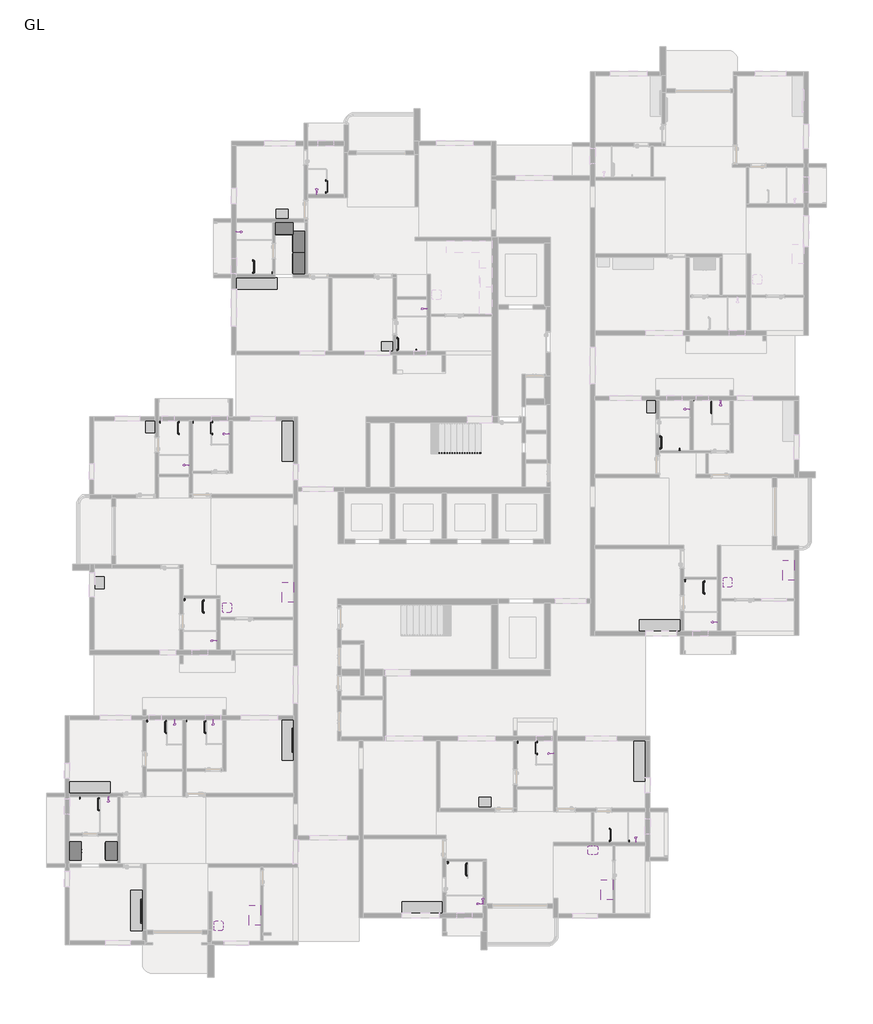
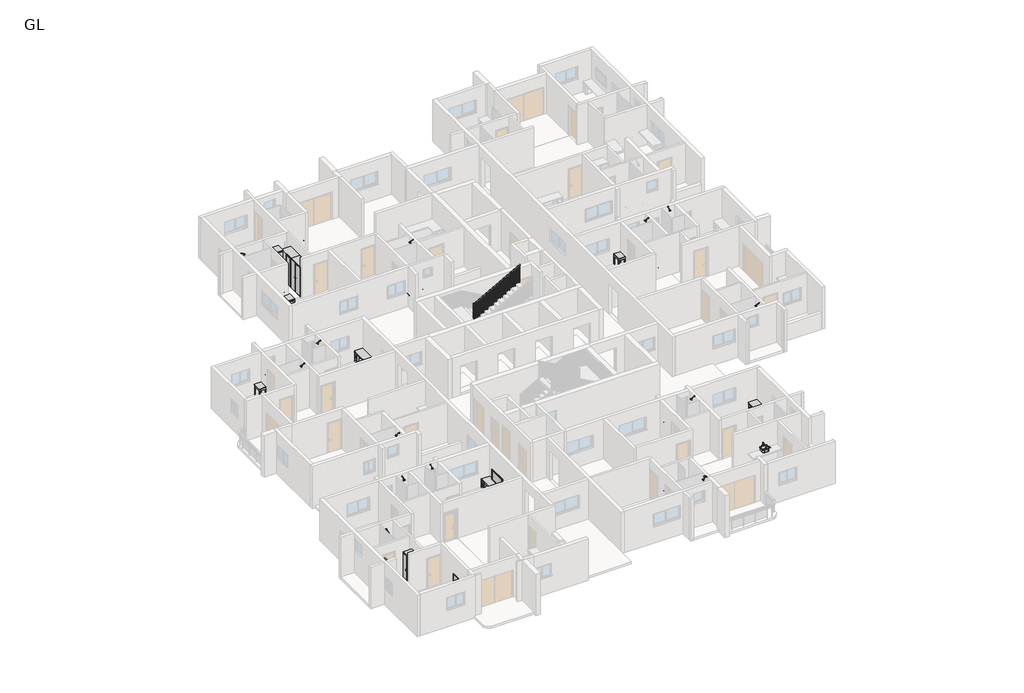
# One storey, part 13 of 14: 50 flow terminals, 23 furniture elements, 4 proxies, 1 railing.
"""IFC4 building model written with IfcOpenShell, lengths in millimetres."""

from ifc_helpers import new_model, si_unit, frame, origin, place, context, project, spatial, polyline, outline, extrude, faceted_brep, transform, mapped, element, save
from components import cook_top_2_0915_x_500mm_892363c5, flow_terminal_f629513f, grab_rail_horizontal_grab_bar_horizontal_f73a8c0c, grab_rail_vertical_grab_rail_vertical_969059c8, plumbing_fixtures_shower_head_metal_shower_head_9404fff0, furniture_8acf2248, escritorio_de_estudiante_de_600x740mm_600_x_460_x_740mm_3f482482, furniture_0b97a49d, furniture_eb486d47, wardrobe_family_wardrobe_large_408d0eaf, wardrobe_family_wardrobe_small_46214fc7

model = new_model("IFC4")

# Units and contexts
model_context = context("Model", 3, world=origin())
ifc_project = project(units=[si_unit("LENGTHUNIT", "METRE", prefix="MILLI")], contexts=[model_context])

# Site, building, storey
site = spatial("IfcSite", under=ifc_project)
building = spatial("IfcBuilding", under=site)
storey = spatial("IfcBuildingStorey", under=building, Name="GL", Elevation=0.0)

# Proxies
placement = place(None, origin())
cook_top_2_0915_x_500mm_shape = cook_top_2_0915_x_500mm_892363c5(model_context)
element("IfcBuildingElementProxy", 1, Name="Cook_Top_(2) : 0915 x 500mm", ObjectType="Cook_Top_(2) : 0915 x 500mm", at=placement, inside=storey, context=model_context, shape_type="MappedRepresentation", body=[
    mapped(cook_top_2_0915_x_500mm_shape, transform((-7432.3172689, 57616.4127724, 457.2), x_axis=(0.0, 1.0, 0.0), y_axis=(-1.0, 0.0, 0.0), z_axis=(0.0, 0.0, 1.0))),
])
element("IfcBuildingElementProxy", 2, Name="Cook_Top_(2) : 0915 x 500mm", ObjectType="Cook_Top_(2) : 0915 x 500mm", at=placement, inside=storey, context=model_context, shape_type="MappedRepresentation", body=[
    mapped(cook_top_2_0915_x_500mm_shape, transform((10113.003694, 58890.1105424, 457.2), x_axis=(0.0, 1.0, 0.0), y_axis=(-1.0, 0.0, 0.0), z_axis=(0.0, 0.0, 1.0))),
])
element("IfcBuildingElementProxy", 3, Name="Cook_Top_(2) : 0915 x 500mm", ObjectType="Cook_Top_(2) : 0915 x 500mm", at=placement, inside=storey, context=model_context, shape_type="MappedRepresentation", body=[
    mapped(cook_top_2_0915_x_500mm_shape, transform((19166.6969726, 74807.6047412, 457.2), x_axis=(0.0, 1.0, 0.0), y_axis=(-1.0, 0.0, 0.0), z_axis=(0.0, 0.0, 1.0))),
])
element("IfcBuildingElementProxy", 4, Name="Cook_Top_(2) : 0915 x 500mm", ObjectType="Cook_Top_(2) : 0915 x 500mm", at=placement, inside=storey, context=model_context, shape_type="MappedRepresentation", body=[
    mapped(cook_top_2_0915_x_500mm_shape, transform((-5780.9131346, 73713.6131717, 457.2), x_axis=(0.0, 1.0, 0.0), y_axis=(-1.0, 0.0, 0.0), z_axis=(0.0, 0.0, 1.0))),
])

# Flow terminals
flow_terminal_shape = flow_terminal_f629513f(model_context)
element("IfcFlowTerminal", 5, at=placement, inside=storey, context=model_context, shape_type="MappedRepresentation", body=[
    mapped(flow_terminal_shape, transform((-9284.2164285, 57077.0304817, 762.0), x_axis=(0.0, 1.0, 0.0), y_axis=(-1.0, 0.0, 0.0), z_axis=(0.0, 0.0, 1.0))),
])
element("IfcFlowTerminal", 6, at=placement, inside=storey, context=model_context, shape_type="MappedRepresentation", body=[
    mapped(flow_terminal_shape, transform((16090.1365547, 74192.2476782, 762.0), x_axis=(0.0, 1.0, 0.0), y_axis=(-1.0, 0.0, 0.0), z_axis=(0.0, 0.0, 1.0))),
])
element("IfcFlowTerminal", 7, at=placement, inside=storey, context=model_context, shape_type="MappedRepresentation", body=[
    mapped(flow_terminal_shape, transform((-8863.3729222, 72934.9514566, 762.0), x_axis=(0.0, 1.0, 0.0), y_axis=(-1.0, 0.0, 0.0), z_axis=(0.0, 0.0, 1.0))),
])
element("IfcFlowTerminal", 8, at=placement, inside=storey, context=model_context, shape_type="MappedRepresentation", body=[
    mapped(flow_terminal_shape, transform((9390.7046133, 60899.7565929, 762.0), x_axis=(1.0, 0.0, 0.0), y_axis=(0.0, 1.0, 0.0), z_axis=(0.0, 0.0, 1.0))),
])
grab_rail_horizontal_grab_bar_horizontal_shape = grab_rail_horizontal_grab_bar_horizontal_f73a8c0c(model_context)
element("IfcFlowTerminal", 9, ObjectType="Grab Rail - Horizontal : Grab Bar Horizontal", at=placement, inside=storey, context=model_context, shape_type="MappedRepresentation", body=[
    mapped(grab_rail_horizontal_grab_bar_horizontal_shape, transform((-15187.4698866, 64009.4643641, 0.0), x_axis=(0.0, 1.0, 0.0), y_axis=(-1.0, 0.0, 0.0), z_axis=(0.0, 0.0, 1.0))),
])
element("IfcFlowTerminal", 10, ObjectType="Grab Rail - Horizontal : Grab Bar Horizontal", at=placement, inside=storey, context=model_context, shape_type="MappedRepresentation", body=[
    mapped(grab_rail_horizontal_grab_bar_horizontal_shape, transform((-11834.397169, 67857.3290817, 0.0), x_axis=(0.0, 1.0, 0.0), y_axis=(-1.0, 0.0, 0.0), z_axis=(0.0, 0.0, 1.0))),
])
element("IfcFlowTerminal", 11, ObjectType="Grab Rail - Horizontal : Grab Bar Horizontal", at=placement, inside=storey, context=model_context, shape_type="MappedRepresentation", body=[
    mapped(grab_rail_horizontal_grab_bar_horizontal_shape, transform((-9878.597169, 67857.3290817, 0.0), x_axis=(0.0, 1.0, 0.0), y_axis=(-1.0, 0.0, 0.0), z_axis=(0.0, 0.0, 1.0))),
])
element("IfcFlowTerminal", 12, ObjectType="Grab Rail - Horizontal : Grab Bar Horizontal", at=placement, inside=storey, context=model_context, shape_type="MappedRepresentation", body=[
    mapped(grab_rail_horizontal_grab_bar_horizontal_shape, transform((6641.3567087, 66815.1785086, 0.0), x_axis=(0.0, 1.0, 0.0), y_axis=(-1.0, 0.0, 0.0), z_axis=(0.0, 0.0, 1.0))),
])
element("IfcFlowTerminal", 13, ObjectType="Grab Rail - Horizontal : Grab Bar Horizontal", at=placement, inside=storey, context=model_context, shape_type="MappedRepresentation", body=[
    mapped(grab_rail_horizontal_grab_bar_horizontal_shape, transform((10234.603694, 60775.9743275, 0.0), x_axis=(0.0, -1.0, 0.0), y_axis=(1.0, 0.0, 0.0), z_axis=(0.0, 0.0, 1.0))),
])
element("IfcFlowTerminal", 14, ObjectType="Grab Rail - Horizontal : Grab Bar Horizontal", at=placement, inside=storey, context=model_context, shape_type="MappedRepresentation", body=[
    mapped(grab_rail_horizontal_grab_bar_horizontal_shape, transform((3159.1144026, 60758.453971, 0.0), x_axis=(0.0, 1.0, 0.0), y_axis=(-1.0, 0.0, 0.0), z_axis=(0.0, 0.0, 1.0))),
])
element("IfcFlowTerminal", 15, ObjectType="Grab Rail - Horizontal : Grab Bar Horizontal", at=placement, inside=storey, context=model_context, shape_type="MappedRepresentation", body=[
    mapped(grab_rail_horizontal_grab_bar_horizontal_shape, transform((14986.6163556, 74808.9935622, 0.0), x_axis=(0.0, 1.0, 0.0), y_axis=(-1.0, 0.0, 0.0), z_axis=(0.0, 0.0, 1.0))),
])
element("IfcFlowTerminal", 16, ObjectType="Grab Rail - Horizontal : Grab Bar Horizontal", at=placement, inside=storey, context=model_context, shape_type="MappedRepresentation", body=[
    mapped(grab_rail_horizontal_grab_bar_horizontal_shape, transform((12762.5764579, 80324.0622292, 0.0), x_axis=(0.0, -1.0, 0.0), y_axis=(1.0, 0.0, 0.0), z_axis=(0.0, 0.0, 1.0))),
])
element("IfcFlowTerminal", 17, ObjectType="Grab Rail - Horizontal : Grab Bar Horizontal", at=placement, inside=storey, context=model_context, shape_type="MappedRepresentation", body=[
    mapped(grab_rail_horizontal_grab_bar_horizontal_shape, transform((15380.1764579, 83771.3835622, 0.0), x_axis=(0.0, 1.0, 0.0), y_axis=(-1.0, 0.0, 0.0), z_axis=(0.0, 0.0, 1.0))),
])
element("IfcFlowTerminal", 18, ObjectType="Grab Rail - Horizontal : Grab Bar Horizontal", at=placement, inside=storey, context=model_context, shape_type="MappedRepresentation", body=[
    mapped(grab_rail_horizontal_grab_bar_horizontal_shape, transform((-7539.4662192, 89078.9881079, 0.0), x_axis=(0.0, -1.0, 0.0), y_axis=(1.0, 0.0, 0.0), z_axis=(0.0, 0.0, 1.0))),
])
element("IfcFlowTerminal", 19, ObjectType="Grab Rail - Horizontal : Grab Bar Horizontal", at=placement, inside=storey, context=model_context, shape_type="MappedRepresentation", body=[
    mapped(grab_rail_horizontal_grab_bar_horizontal_shape, transform((-353.887999, 85234.2279589, 0.0), x_axis=(0.0, -1.0, 0.0), y_axis=(1.0, 0.0, 0.0), z_axis=(0.0, 0.0, 1.0))),
])
element("IfcFlowTerminal", 20, ObjectType="Grab Rail - Horizontal : Grab Bar Horizontal", at=placement, inside=storey, context=model_context, shape_type="MappedRepresentation", body=[
    mapped(grab_rail_horizontal_grab_bar_horizontal_shape, transform((-3903.094999, 93069.4085634, 0.0), x_axis=(0.0, -1.0, 0.0), y_axis=(1.0, 0.0, 0.0), z_axis=(0.0, 0.0, 1.0))),
])
element("IfcFlowTerminal", 21, ObjectType="Grab Rail - Horizontal : Grab Bar Horizontal", at=placement, inside=storey, context=model_context, shape_type="MappedRepresentation", body=[
    mapped(grab_rail_horizontal_grab_bar_horizontal_shape, transform((-9968.1631346, 73865.6984389, 0.0), x_axis=(0.0, 1.0, 0.0), y_axis=(-1.0, 0.0, 0.0), z_axis=(0.0, 0.0, 1.0))),
])
element("IfcFlowTerminal", 22, ObjectType="Grab Rail - Horizontal : Grab Bar Horizontal", at=placement, inside=storey, context=model_context, shape_type="MappedRepresentation", body=[
    mapped(grab_rail_horizontal_grab_bar_horizontal_shape, transform((-11196.8261346, 82754.8603664, 0.0), x_axis=(0.0, 1.0, 0.0), y_axis=(-1.0, 0.0, 0.0), z_axis=(0.0, 0.0, 1.0))),
])
element("IfcFlowTerminal", 23, ObjectType="Grab Rail - Horizontal : Grab Bar Horizontal", at=placement, inside=storey, context=model_context, shape_type="MappedRepresentation", body=[
    mapped(grab_rail_horizontal_grab_bar_horizontal_shape, transform((-9551.3491346, 82754.8603664, 0.0), x_axis=(0.0, 1.0, 0.0), y_axis=(-1.0, 0.0, 0.0), z_axis=(0.0, 0.0, 1.0))),
])
grab_rail_vertical_grab_rail_vertical_shape = grab_rail_vertical_grab_rail_vertical_969059c8(model_context)
element("IfcFlowTerminal", 24, ObjectType="Grab Rail - Vertical : Grab Rail Vertical", at=placement, inside=storey, context=model_context, shape_type="MappedRepresentation", body=[
    mapped(grab_rail_vertical_grab_rail_vertical_shape, transform((-17013.2655531, 63531.8006976, 0.0), x_axis=(-1.0, 0.0, 0.0), y_axis=(0.0, -1.0, 0.0), z_axis=(0.0, 0.0, 1.0))),
])
element("IfcFlowTerminal", 25, ObjectType="Grab Rail - Vertical : Grab Rail Vertical", at=placement, inside=storey, context=model_context, shape_type="MappedRepresentation", body=[
    mapped(grab_rail_vertical_grab_rail_vertical_shape, transform((-13660.1928355, 67367.4734152, 0.0), x_axis=(-1.0, 0.0, 0.0), y_axis=(0.0, -1.0, 0.0), z_axis=(0.0, 0.0, 1.0))),
])
element("IfcFlowTerminal", 26, ObjectType="Grab Rail - Vertical : Grab Rail Vertical", at=placement, inside=storey, context=model_context, shape_type="MappedRepresentation", body=[
    mapped(grab_rail_vertical_grab_rail_vertical_shape, transform((-11704.3928355, 67367.4734152, 0.0), x_axis=(-1.0, 0.0, 0.0), y_axis=(0.0, -1.0, 0.0), z_axis=(0.0, 0.0, 1.0))),
])
element("IfcFlowTerminal", 27, ObjectType="Grab Rail - Vertical : Grab Rail Vertical", at=placement, inside=storey, context=model_context, shape_type="MappedRepresentation", body=[
    mapped(grab_rail_vertical_grab_rail_vertical_shape, transform((4815.5610422, 66317.7028421, 0.0), x_axis=(-1.0, 0.0, 0.0), y_axis=(0.0, -1.0, 0.0), z_axis=(0.0, 0.0, 1.0))),
])
element("IfcFlowTerminal", 28, ObjectType="Grab Rail - Vertical : Grab Rail Vertical", at=placement, inside=storey, context=model_context, shape_type="MappedRepresentation", body=[
    mapped(grab_rail_vertical_grab_rail_vertical_shape, transform((12060.3993605, 61253.637994, 0.0), x_axis=(1.0, 0.0, 0.0), y_axis=(0.0, 1.0, 0.0), z_axis=(0.0, 0.0, 1.0))),
])
element("IfcFlowTerminal", 29, ObjectType="Grab Rail - Vertical : Grab Rail Vertical", at=placement, inside=storey, context=model_context, shape_type="MappedRepresentation", body=[
    mapped(grab_rail_vertical_grab_rail_vertical_shape, transform((1333.3187361, 60310.5083045, 0.0), x_axis=(-1.0, 0.0, 0.0), y_axis=(0.0, -1.0, 0.0), z_axis=(0.0, 0.0, 1.0))),
])
element("IfcFlowTerminal", 30, ObjectType="Grab Rail - Vertical : Grab Rail Vertical", at=placement, inside=storey, context=model_context, shape_type="MappedRepresentation", body=[
    mapped(grab_rail_vertical_grab_rail_vertical_shape, transform((13160.8206891, 74361.0478957, 0.0), x_axis=(-1.0, 0.0, 0.0), y_axis=(0.0, -1.0, 0.0), z_axis=(0.0, 0.0, 1.0))),
])
element("IfcFlowTerminal", 31, ObjectType="Grab Rail - Vertical : Grab Rail Vertical", at=placement, inside=storey, context=model_context, shape_type="MappedRepresentation", body=[
    mapped(grab_rail_vertical_grab_rail_vertical_shape, transform((14588.3721244, 80772.0078957, 0.0), x_axis=(1.0, 0.0, 0.0), y_axis=(0.0, 1.0, 0.0), z_axis=(0.0, 0.0, 1.0))),
])
element("IfcFlowTerminal", 32, ObjectType="Grab Rail - Vertical : Grab Rail Vertical", at=placement, inside=storey, context=model_context, shape_type="MappedRepresentation", body=[
    mapped(grab_rail_vertical_grab_rail_vertical_shape, transform((13554.3807914, 83273.9078957, 0.0), x_axis=(-1.0, 0.0, 0.0), y_axis=(0.0, -1.0, 0.0), z_axis=(0.0, 0.0, 1.0))),
])
element("IfcFlowTerminal", 33, ObjectType="Grab Rail - Vertical : Grab Rail Vertical", at=placement, inside=storey, context=model_context, shape_type="MappedRepresentation", body=[
    mapped(grab_rail_vertical_grab_rail_vertical_shape, transform((-5713.6705527, 89556.6517744, 0.0), x_axis=(1.0, 0.0, 0.0), y_axis=(0.0, 1.0, 0.0), z_axis=(0.0, 0.0, 1.0))),
])
element("IfcFlowTerminal", 34, ObjectType="Grab Rail - Vertical : Grab Rail Vertical", at=placement, inside=storey, context=model_context, shape_type="MappedRepresentation", body=[
    mapped(grab_rail_vertical_grab_rail_vertical_shape, transform((1471.9076675, 85711.8916254, 0.0), x_axis=(1.0, 0.0, 0.0), y_axis=(0.0, 1.0, 0.0), z_axis=(0.0, 0.0, 1.0))),
])
element("IfcFlowTerminal", 35, ObjectType="Grab Rail - Vertical : Grab Rail Vertical", at=placement, inside=storey, context=model_context, shape_type="MappedRepresentation", body=[
    mapped(grab_rail_vertical_grab_rail_vertical_shape, transform((-2077.2993325, 93547.0722299, 0.0), x_axis=(1.0, 0.0, 0.0), y_axis=(0.0, 1.0, 0.0), z_axis=(0.0, 0.0, 1.0))),
])
element("IfcFlowTerminal", 36, ObjectType="Grab Rail - Vertical : Grab Rail Vertical", at=placement, inside=storey, context=model_context, shape_type="MappedRepresentation", body=[
    mapped(grab_rail_vertical_grab_rail_vertical_shape, transform((-11793.9588011, 73417.7527724, 0.0), x_axis=(-1.0, 0.0, 0.0), y_axis=(0.0, -1.0, 0.0), z_axis=(0.0, 0.0, 1.0))),
])
element("IfcFlowTerminal", 37, ObjectType="Grab Rail - Vertical : Grab Rail Vertical", at=placement, inside=storey, context=model_context, shape_type="MappedRepresentation", body=[
    mapped(grab_rail_vertical_grab_rail_vertical_shape, transform((-13022.6218011, 82265.0046999, 0.0), x_axis=(-1.0, 0.0, 0.0), y_axis=(0.0, -1.0, 0.0), z_axis=(0.0, 0.0, 1.0))),
])
element("IfcFlowTerminal", 38, ObjectType="Grab Rail - Vertical : Grab Rail Vertical", at=placement, inside=storey, context=model_context, shape_type="MappedRepresentation", body=[
    mapped(grab_rail_vertical_grab_rail_vertical_shape, transform((-11377.1448011, 82265.0046999, 0.0), x_axis=(-1.0, 0.0, 0.0), y_axis=(0.0, -1.0, 0.0), z_axis=(0.0, 0.0, 1.0))),
])
plumbing_fixtures_shower_head_metal_shower_head_shape = plumbing_fixtures_shower_head_metal_shower_head_9404fff0(model_context)
element("IfcFlowTerminal", 39, ObjectType="Plumbing_Fixtures_Shower_Head : Metal_Shower_Head", at=placement, inside=storey, context=model_context, shape_type="MappedRepresentation", body=[
    mapped(plumbing_fixtures_shower_head_metal_shower_head_shape, transform((-14730.2698866, 63531.8006976, 914.4), x_axis=(-1.0, 0.0, 0.0), y_axis=(0.0, -1.0, 0.0), z_axis=(0.0, 0.0, 1.0))),
])
element("IfcFlowTerminal", 40, ObjectType="Plumbing_Fixtures_Shower_Head : Metal_Shower_Head", at=placement, inside=storey, context=model_context, shape_type="MappedRepresentation", body=[
    mapped(plumbing_fixtures_shower_head_metal_shower_head_shape, transform((-11433.7122852, 67367.4734152, 1219.2), x_axis=(-1.0, 0.0, 0.0), y_axis=(0.0, -1.0, 0.0), z_axis=(0.0, 0.0, 1.0))),
])
element("IfcFlowTerminal", 41, ObjectType="Plumbing_Fixtures_Shower_Head : Metal_Shower_Head", at=placement, inside=storey, context=model_context, shape_type="MappedRepresentation", body=[
    mapped(plumbing_fixtures_shower_head_metal_shower_head_shape, transform((-9514.2506601, 67367.4734152, 1369.1616), x_axis=(-1.0, 0.0, 0.0), y_axis=(0.0, -1.0, 0.0), z_axis=(0.0, 0.0, 1.0))),
])
element("IfcFlowTerminal", 42, ObjectType="Plumbing_Fixtures_Shower_Head : Metal_Shower_Head", at=placement, inside=storey, context=model_context, shape_type="MappedRepresentation", body=[
    mapped(plumbing_fixtures_shower_head_metal_shower_head_shape, transform((3929.8233567, 58192.7833045, 1369.1616), x_axis=(0.0, 1.0, 0.0), y_axis=(-1.0, 0.0, 0.0), z_axis=(0.0, 0.0, 1.0))),
])
element("IfcFlowTerminal", 43, ObjectType="Plumbing_Fixtures_Shower_Head : Metal_Shower_Head", at=placement, inside=storey, context=model_context, shape_type="MappedRepresentation", body=[
    mapped(plumbing_fixtures_shower_head_metal_shower_head_shape, transform((7449.877694, 65683.1028421, 1369.1616), x_axis=(0.0, 1.0, 0.0), y_axis=(-1.0, 0.0, 0.0), z_axis=(0.0, 0.0, 1.0))),
])
element("IfcFlowTerminal", 44, ObjectType="Plumbing_Fixtures_Shower_Head : Metal_Shower_Head", at=placement, inside=storey, context=model_context, shape_type="MappedRepresentation", body=[
    mapped(plumbing_fixtures_shower_head_metal_shower_head_shape, transform((11556.803694, 61253.637994, 1219.2), x_axis=(1.0, 0.0, 0.0), y_axis=(0.0, 1.0, 0.0), z_axis=(0.0, 0.0, 1.0))),
])
element("IfcFlowTerminal", 45, ObjectType="Plumbing_Fixtures_Shower_Head : Metal_Shower_Head", at=placement, inside=storey, context=model_context, shape_type="MappedRepresentation", body=[
    mapped(plumbing_fixtures_shower_head_metal_shower_head_shape, transform((3929.8233567, 58192.7833045, 1369.1616), x_axis=(1.0, 0.0, 0.0), y_axis=(0.0, 1.0, 0.0), z_axis=(0.0, 0.0, 1.0))),
])
element("IfcFlowTerminal", 46, ObjectType="Plumbing_Fixtures_Shower_Head : Metal_Shower_Head", at=placement, inside=storey, context=model_context, shape_type="MappedRepresentation", body=[
    mapped(plumbing_fixtures_shower_head_metal_shower_head_shape, transform((15615.0862029, 72230.5478957, 1219.2), x_axis=(0.0, 1.0, 0.0), y_axis=(-1.0, 0.0, 0.0), z_axis=(0.0, 0.0, 1.0))),
])
element("IfcFlowTerminal", 47, ObjectType="Plumbing_Fixtures_Shower_Head : Metal_Shower_Head", at=placement, inside=storey, context=model_context, shape_type="MappedRepresentation", body=[
    mapped(plumbing_fixtures_shower_head_metal_shower_head_shape, transform((14242.1264579, 82842.1078957, 1369.1616), x_axis=(0.0, 1.0, 0.0), y_axis=(-1.0, 0.0, 0.0), z_axis=(0.0, 0.0, 1.0))),
])
element("IfcFlowTerminal", 48, ObjectType="Plumbing_Fixtures_Shower_Head : Metal_Shower_Head", at=placement, inside=storey, context=model_context, shape_type="MappedRepresentation", body=[
    mapped(plumbing_fixtures_shower_head_metal_shower_head_shape, transform((15781.1124579, 83273.9078957, 1369.1616), x_axis=(-1.0, 0.0, 0.0), y_axis=(0.0, -1.0, 0.0), z_axis=(0.0, 0.0, 1.0))),
])
element("IfcFlowTerminal", 49, ObjectType="Plumbing_Fixtures_Shower_Head : Metal_Shower_Head", at=placement, inside=storey, context=model_context, shape_type="MappedRepresentation", body=[
    mapped(plumbing_fixtures_shower_head_metal_shower_head_shape, transform((-8359.394999, 91667.112129, 1369.1616), x_axis=(0.0, -1.0, 0.0), y_axis=(1.0, 0.0, 0.0), z_axis=(0.0, 0.0, 1.0))),
])
element("IfcFlowTerminal", 50, ObjectType="Plumbing_Fixtures_Shower_Head : Metal_Shower_Head", at=placement, inside=storey, context=model_context, shape_type="MappedRepresentation", body=[
    mapped(plumbing_fixtures_shower_head_metal_shower_head_shape, transform((1156.969001, 87839.1416254, 1369.1616), x_axis=(0.0, 1.0, 0.0), y_axis=(-1.0, 0.0, 0.0), z_axis=(0.0, 0.0, 1.0))),
])
element("IfcFlowTerminal", 51, ObjectType="Plumbing_Fixtures_Shower_Head : Metal_Shower_Head", at=placement, inside=storey, context=model_context, shape_type="MappedRepresentation", body=[
    mapped(plumbing_fixtures_shower_head_metal_shower_head_shape, transform((-4348.0802192, 93547.0722299, 1219.2), x_axis=(1.0, 0.0, 0.0), y_axis=(0.0, 1.0, 0.0), z_axis=(0.0, 0.0, 1.0))),
])
element("IfcFlowTerminal", 52, ObjectType="Plumbing_Fixtures_Shower_Head : Metal_Shower_Head", at=placement, inside=storey, context=model_context, shape_type="MappedRepresentation", body=[
    mapped(plumbing_fixtures_shower_head_metal_shower_head_shape, transform((-9336.8491346, 71303.2027724, 1219.2), x_axis=(0.0, 1.0, 0.0), y_axis=(-1.0, 0.0, 0.0), z_axis=(0.0, 0.0, 1.0))),
])
element("IfcFlowTerminal", 53, ObjectType="Plumbing_Fixtures_Shower_Head : Metal_Shower_Head", at=placement, inside=storey, context=model_context, shape_type="MappedRepresentation", body=[
    mapped(plumbing_fixtures_shower_head_metal_shower_head_shape, transform((-8724.3991708, 81605.0046999, 1369.1616), x_axis=(0.0, 1.0, 0.0), y_axis=(-1.0, 0.0, 0.0), z_axis=(0.0, 0.0, 1.0))),
])
element("IfcFlowTerminal", 54, ObjectType="Plumbing_Fixtures_Shower_Head : Metal_Shower_Head", at=placement, inside=storey, context=model_context, shape_type="MappedRepresentation", body=[
    mapped(plumbing_fixtures_shower_head_metal_shower_head_shape, transform((-10721.1491346, 80052.6646999, 1369.1616), x_axis=(0.0, 1.0, 0.0), y_axis=(-1.0, 0.0, 0.0), z_axis=(0.0, 0.0, 1.0))),
])

# Furniture
furniture_shape = furniture_8acf2248(model_context)
element("IfcFurniture", 55, at=placement, inside=storey, context=model_context, shape_type="MappedRepresentation", body=[
    mapped(furniture_shape, transform((-13033.6798866, 58878.7934152, 149.9616), x_axis=(0.0, -1.0, 0.0), y_axis=(1.0, 0.0, 0.0), z_axis=(0.0, 0.0, 1.0))),
])
element("IfcFurniture", 56, at=placement, inside=storey, context=model_context, shape_type="MappedRepresentation", body=[
    mapped(furniture_shape, transform((-5492.8131346, 67367.4734152, 0.0), x_axis=(0.0, -1.0, 0.0), y_axis=(1.0, 0.0, 0.0), z_axis=(0.0, 0.0, 1.0))),
])
element("IfcFurniture", 57, at=placement, inside=storey, context=model_context, shape_type="MappedRepresentation", body=[
    mapped(furniture_shape, transform((-14654.0698866, 63705.5366976, 0.0), x_axis=(-1.0, 0.0, 0.0), y_axis=(0.0, -1.0, 0.0), z_axis=(0.0, 0.0, 1.0))),
])
element("IfcFurniture", 58, at=placement, inside=storey, context=model_context, shape_type="MappedRepresentation", body=[
    mapped(furniture_shape, transform((1930.5893567, 57723.2565193, 149.9616), x_axis=(-1.0, 0.0, 0.0), y_axis=(0.0, -1.0, 0.0), z_axis=(0.0, 0.0, 1.0))),
])
element("IfcFurniture", 59, at=placement, inside=storey, context=model_context, shape_type="MappedRepresentation", body=[
    mapped(furniture_shape, transform((12039.403694, 66317.7028421, 0.0), x_axis=(0.0, -1.0, 0.0), y_axis=(1.0, 0.0, 0.0), z_axis=(0.0, 0.0, 1.0))),
])
element("IfcFurniture", 60, at=placement, inside=storey, context=model_context, shape_type="MappedRepresentation", body=[
    mapped(furniture_shape, transform((13770.0803556, 71762.6278957, 149.9616), x_axis=(-1.0, 0.0, 0.0), y_axis=(0.0, -1.0, 0.0), z_axis=(0.0, 0.0, 1.0))),
])
element("IfcFurniture", 61, at=placement, inside=storey, context=model_context, shape_type="MappedRepresentation", body=[
    mapped(furniture_shape, transform((-8359.394999, 89382.9157744, 0.0), x_axis=(1.0, 0.0, 0.0), y_axis=(0.0, 1.0, 0.0), z_axis=(0.0, 0.0, 1.0))),
])
element("IfcFurniture", 62, at=placement, inside=storey, context=model_context, shape_type="MappedRepresentation", body=[
    mapped(furniture_shape, transform((-5492.8131346, 82265.0046999, 149.9616), x_axis=(0.0, -1.0, 0.0), y_axis=(1.0, 0.0, 0.0), z_axis=(0.0, 0.0, 1.0))),
])
escritorio_de_estudiante_de_600x740mm_600_x_460_x_740mm_shape = escritorio_de_estudiante_de_600x740mm_600_x_460_x_740mm_3f482482(model_context)
element("IfcFurniture", 63, ObjectType="Escritorio_de_estudiante_de_600x740mm : 600 x 460 x 740mm", at=placement, inside=storey, context=model_context, shape_type="MappedRepresentation", body=[
    mapped(escritorio_de_estudiante_de_600x740mm_600_x_460_x_740mm_shape, transform((4029.513694, 63269.7028421, 149.9616), x_axis=(1.0, 0.0, 0.0), y_axis=(0.0, 1.0, 0.0), z_axis=(0.0, 0.0, 1.0))),
])
element("IfcFurniture", 64, ObjectType="Escritorio_de_estudiante_de_600x740mm : 600 x 460 x 740mm", at=placement, inside=storey, context=model_context, shape_type="MappedRepresentation", body=[
    mapped(escritorio_de_estudiante_de_600x740mm_600_x_460_x_740mm_shape, transform((12327.5569726, 82969.1078957, 149.9616), x_axis=(0.0, 1.0, 0.0), y_axis=(-1.0, 0.0, 0.0), z_axis=(0.0, 0.0, 1.0))),
])
element("IfcFurniture", 65, ObjectType="Escritorio_de_estudiante_de_600x740mm : 600 x 460 x 740mm", at=placement, inside=storey, context=model_context, shape_type="MappedRepresentation", body=[
    mapped(escritorio_de_estudiante_de_600x740mm_600_x_460_x_740mm_shape, transform((-6071.2162192, 92560.5362299, 149.9616), x_axis=(1.0, 0.0, 0.0), y_axis=(0.0, 1.0, 0.0), z_axis=(0.0, 0.0, 1.0))),
])
element("IfcFurniture", 66, ObjectType="Escritorio_de_estudiante_de_600x740mm : 600 x 460 x 740mm", at=placement, inside=storey, context=model_context, shape_type="MappedRepresentation", body=[
    mapped(escritorio_de_estudiante_de_600x740mm_600_x_460_x_740mm_shape, transform((-824.230999, 85959.5416254, 149.9616), x_axis=(1.0, 0.0, 0.0), y_axis=(0.0, 1.0, 0.0), z_axis=(0.0, 0.0, 1.0))),
])
element("IfcFurniture", 67, ObjectType="Escritorio_de_estudiante_de_600x740mm : 600 x 460 x 740mm", at=placement, inside=storey, context=model_context, shape_type="MappedRepresentation", body=[
    mapped(escritorio_de_estudiante_de_600x740mm_600_x_460_x_740mm_shape, transform((-12639.1031346, 81960.2046999, 149.9616), x_axis=(0.0, 1.0, 0.0), y_axis=(-1.0, 0.0, 0.0), z_axis=(0.0, 0.0, 1.0))),
])
element("IfcFurniture", 68, ObjectType="Escritorio_de_estudiante_de_600x740mm : 600 x 460 x 740mm", at=placement, inside=storey, context=model_context, shape_type="MappedRepresentation", body=[
    mapped(escritorio_de_estudiante_de_600x740mm_600_x_460_x_740mm_shape, transform((-15172.7531346, 74191.1827724, 149.9616), x_axis=(0.0, 1.0, 0.0), y_axis=(-1.0, 0.0, 0.0), z_axis=(0.0, 0.0, 1.0))),
])
furniture_2_shape = furniture_0b97a49d(model_context)
element("IfcFurniture", 69, ObjectType="Furniture_TV_Plasma : 42\"", at=placement, inside=storey, context=model_context, shape_type="MappedRepresentation", body=[
    mapped(furniture_2_shape, transform((-5492.8131346, 80928.9646999, 0.0), x_axis=(0.0, -1.0, 0.0), y_axis=(1.0, 0.0, 0.0), z_axis=(0.0, 0.0, 1.0))),
])
furniture_3_shape = furniture_eb486d47(model_context)
element("IfcFurniture", 70, ObjectType="Furniture_TV_Plasma : 50\"", at=placement, inside=storey, context=model_context, shape_type="MappedRepresentation", body=[
    mapped(furniture_3_shape, transform((-13033.6798866, 57881.8434152, 1066.8), x_axis=(0.0, -1.0, 0.0), y_axis=(1.0, 0.0, 0.0), z_axis=(0.0, 0.0, 1.0))),
])
element("IfcFurniture", 71, ObjectType="Furniture_TV_Plasma : 50\"", at=placement, inside=storey, context=model_context, shape_type="MappedRepresentation", body=[
    mapped(furniture_3_shape, transform((-5492.8131346, 66400.7487724, 762.0), x_axis=(0.0, -1.0, 0.0), y_axis=(1.0, 0.0, 0.0), z_axis=(0.0, 0.0, 1.0))),
])
element("IfcFurniture", 72, ObjectType="Furniture_TV_Plasma : 50\"", at=placement, inside=storey, context=model_context, shape_type="MappedRepresentation", body=[
    mapped(furniture_3_shape, transform((-5492.8131346, 81017.8646999, 0.0), x_axis=(0.0, -1.0, 0.0), y_axis=(1.0, 0.0, 0.0), z_axis=(0.0, 0.0, 1.0))),
])
wardrobe_family_wardrobe_large_shape = wardrobe_family_wardrobe_large_408d0eaf(model_context)
element("IfcFurniture", 73, ObjectType="Wardrobe-Family : Wardrobe - Large", at=placement, inside=storey, context=model_context, shape_type="MappedRepresentation", body=[
    mapped(wardrobe_family_wardrobe_large_shape, transform((-5233.0162192, 90090.0517744, 149.9616), x_axis=(0.0, -1.0, 0.0), y_axis=(1.0, 0.0, 0.0), z_axis=(0.0, 0.0, 1.0))),
])
element("IfcFurniture", 74, ObjectType="Wardrobe-Family : Wardrobe - Large", at=placement, inside=storey, context=model_context, shape_type="MappedRepresentation", body=[
    mapped(wardrobe_family_wardrobe_large_shape, transform((-5233.0162192, 91156.8517744, 149.9616), x_axis=(0.0, -1.0, 0.0), y_axis=(1.0, 0.0, 0.0), z_axis=(0.0, 0.0, 1.0))),
])
wardrobe_family_wardrobe_small_shape = wardrobe_family_wardrobe_small_46214fc7(model_context)
element("IfcFurniture", 75, ObjectType="Wardrobe-Family : Wardrobe - Small", at=placement, inside=storey, context=model_context, shape_type="MappedRepresentation", body=[
    mapped(wardrobe_family_wardrobe_small_shape, transform((-16408.0698866, 60826.4695727, 149.9616), x_axis=(0.0, 1.0, 0.0), y_axis=(-1.0, 0.0, 0.0), z_axis=(0.0, 0.0, 1.0))),
])
element("IfcFurniture", 76, ObjectType="Wardrobe-Family : Wardrobe - Small", at=placement, inside=storey, context=model_context, shape_type="MappedRepresentation", body=[
    mapped(wardrobe_family_wardrobe_small_shape, transform((-14570.4407376, 60826.4695727, 149.9616), x_axis=(0.0, -1.0, 0.0), y_axis=(1.0, 0.0, 0.0), z_axis=(0.0, 0.0, 1.0))),
])
element("IfcFurniture", 77, ObjectType="Wardrobe-Family : Wardrobe - Small", at=placement, inside=storey, context=model_context, shape_type="MappedRepresentation", body=[
    mapped(wardrobe_family_wardrobe_small_shape, transform((-5995.0162192, 91844.912129, 149.9616), x_axis=(1.0, 0.0, 0.0), y_axis=(0.0, 1.0, 0.0), z_axis=(0.0, 0.0, 1.0))),
])

# Railing
element("IfcRailing", 78, ObjectType="1100mm", at=placement, inside=storey, context=model_context, shape_type="SolidModel", body=[
    faceted_brep([(3830.8691495, 80618.5615983, 1266.6666667), (3830.8691495, 80618.5615983, 1209.5255958), (3830.8691495, 80668.5615983, 1209.5255958), (3830.8691495, 80668.5615983, 1266.6666667), (1194.0191495, 80618.5615983, 2725.3972352), (1144.0191495, 80618.5615983, 2695.9166412), (1144.0191495, 80668.5615983, 2695.9166412), (1194.0191495, 80668.5615983, 2725.3972352), (1194.0191495, 80618.5615983, 2766.6666667), (1144.0191495, 80618.5615983, 2716.6666667), (1144.0191495, 80668.5615983, 2716.6666667), (1194.0191495, 80668.5615983, 2766.6666667), (1119.0191495, 80618.5615983, 2766.6666667), (1119.0191495, 80618.5615983, 2716.6666667), (1069.0191495, 80668.5615983, 2716.6666667), (1069.0191495, 80668.5615983, 2766.6666667), (1119.0191495, 80543.5615983, 2766.6666667), (1119.0191495, 80543.5615983, 2716.6666667), (1069.0191495, 80543.5615983, 2716.6666667), (1069.0191495, 80543.5615983, 2766.6666667), (1119.0191495, 80493.4950959, 2766.6666667), (1069.0191495, 80493.4950959, 2766.6666667), (1069.0191495, 80443.4950959, 2716.6666667), (1119.0191495, 80443.4950959, 2716.6666667)], [[[0, 1, 2, 3]], [[1, 0, 4, 5]], [[2, 1, 5, 6]], [[3, 2, 6, 7]], [[0, 3, 7, 4]], [[5, 4, 8, 9]], [[6, 5, 9, 10]], [[7, 6, 10, 11]], [[4, 7, 11, 8]], [[9, 8, 12, 13]], [[10, 9, 13, 14]], [[11, 10, 14, 15]], [[8, 11, 15, 12]], [[13, 12, 16, 17]], [[14, 13, 17, 18]], [[15, 14, 18, 19]], [[12, 15, 19, 16]], [[20, 21, 22, 23]], [[17, 16, 20, 23]], [[18, 17, 23, 22]], [[19, 18, 22, 21]], [[16, 19, 21, 20]]]),
    faceted_brep([(1119.0191495, 80493.4950959, 2766.6666667), (1119.0191495, 80443.4950959, 2716.6666667), (1069.0191495, 80443.4950959, 2716.6666667), (1069.0191495, 80493.4950959, 2766.6666667), (1119.0191495, 80493.4950959, 2875.9102109), (1069.0191495, 80493.4950959, 2905.3272998), (1069.0191495, 80443.4950959, 2905.3272998), (1119.0191495, 80443.4950959, 2875.9102109)], [[[0, 1, 2, 3]], [[4, 5, 6, 7]], [[1, 0, 4, 7]], [[2, 1, 7, 6]], [[3, 2, 6, 5]], [[0, 3, 5, 4]]]),
    faceted_brep([(1069.0191495, 80493.4950959, 2905.3272998), (1119.0191495, 80493.4950959, 2875.9102109), (1119.0191495, 80443.4950959, 2875.9102109), (1069.0191495, 80443.4950959, 2905.3272998), (4118.7728387, 80493.4950959, 4600.0), (4118.7728387, 80443.4950959, 4600.0), (4118.7728387, 80443.4950959, 4542.7991476), (4118.7728387, 80493.4950959, 4542.7991476)], [[[0, 1, 2, 3]], [[4, 5, 6, 7]], [[1, 0, 4, 7]], [[2, 1, 7, 6]], [[3, 2, 6, 5]], [[0, 3, 5, 4]]]),
    extrude(outline(polyline([(3333.3333333, 4019.0191495), (3333.3333333, 4044.0191495), (4501.2603713, 4044.0191495), (4487.3684896, 4019.0191495), (3333.3333333, 4019.0191495)])), frame((0.0, 80455.9950959, 0.0), z_axis=(0.0, 1.0, 0.0), x_axis=(0.0, 0.0, 1.0)), (0.0, 0.0, 1.0), 25.0),
    extrude(outline(polyline([(3333.3333333, 3894.0191495), (3333.3333333, 3919.0191495), (4431.8009628, 3919.0191495), (4417.9090811, 3894.0191495), (3333.3333333, 3894.0191495)])), frame((0.0, 80455.9950959, 0.0), z_axis=(0.0, 1.0, 0.0), x_axis=(0.0, 0.0, 1.0)), (0.0, 0.0, 1.0), 25.0),
    extrude(outline(polyline([(3166.6666667, 3769.0191495), (3166.6666667, 3794.0191495), (4362.3415542, 3794.0191495), (4348.4496725, 3769.0191495), (3166.6666667, 3769.0191495)])), frame((0.0, 80455.9950959, 0.0), z_axis=(0.0, 1.0, 0.0), x_axis=(0.0, 0.0, 1.0)), (0.0, 0.0, 1.0), 25.0),
    extrude(outline(polyline([(3166.6666667, 3644.0191495), (3166.6666667, 3669.0191495), (4292.8821456, 3669.0191495), (4278.9902639, 3644.0191495), (3166.6666667, 3644.0191495)])), frame((0.0, 80455.9950959, 0.0), z_axis=(0.0, 1.0, 0.0), x_axis=(0.0, 0.0, 1.0)), (0.0, 0.0, 1.0), 25.0),
    extrude(outline(polyline([(3166.6666667, 3519.0191495), (3166.6666667, 3544.0191495), (4223.3558342, 3544.0191495), (4209.5255958, 3519.0191495), (3166.6666667, 3519.0191495)])), frame((0.0, 80455.9950959, 0.0), z_axis=(0.0, 1.0, 0.0), x_axis=(0.0, 0.0, 1.0)), (0.0, 0.0, 1.0), 25.0),
    extrude(outline(polyline([(3000.0, 3394.0191495), (3000.0, 3419.0191495), (4153.9633285, 3419.0191495), (4140.0714468, 3394.0191495), (3000.0, 3394.0191495)])), frame((0.0, 80455.9950959, 0.0), z_axis=(0.0, 1.0, 0.0), x_axis=(0.0, 0.0, 1.0)), (0.0, 0.0, 1.0), 25.0),
    extrude(outline(polyline([(3000.0, 3269.0191495), (3000.0, 3294.0191495), (4084.3496444, 3294.0191495), (4070.519406, 3269.0191495), (3000.0, 3269.0191495)])), frame((0.0, 80455.9950959, 0.0), z_axis=(0.0, 1.0, 0.0), x_axis=(0.0, 0.0, 1.0)), (0.0, 0.0, 1.0), 25.0),
    extrude(outline(polyline([(2833.3333333, 3144.0191495), (2833.3333333, 3169.0191495), (4015.0445114, 3169.0191495), (4001.1526297, 3144.0191495), (2833.3333333, 3144.0191495)])), frame((0.0, 80455.9950959, 0.0), z_axis=(0.0, 1.0, 0.0), x_axis=(0.0, 0.0, 1.0)), (0.0, 0.0, 1.0), 25.0),
    extrude(outline(polyline([(2833.3333333, 3019.0191495), (2833.3333333, 3044.0191495), (3945.5851028, 3044.0191495), (3931.6932211, 3019.0191495), (2833.3333333, 3019.0191495)])), frame((0.0, 80455.9950959, 0.0), z_axis=(0.0, 1.0, 0.0), x_axis=(0.0, 0.0, 1.0)), (0.0, 0.0, 1.0), 25.0),
    extrude(outline(polyline([(2666.6666667, 2894.0191495), (2666.6666667, 2919.0191495), (3876.132481, 2919.0191495), (3862.2405993, 2894.0191495), (2666.6666667, 2894.0191495)])), frame((0.0, 80455.9950959, 0.0), z_axis=(0.0, 1.0, 0.0), x_axis=(0.0, 0.0, 1.0)), (0.0, 0.0, 1.0), 25.0),
    extrude(outline(polyline([(2666.6666667, 2769.0191495), (2666.6666667, 2794.0191495), (3806.6662857, 2794.0191495), (3792.774404, 2769.0191495), (2666.6666667, 2769.0191495)])), frame((0.0, 80455.9950959, 0.0), z_axis=(0.0, 1.0, 0.0), x_axis=(0.0, 0.0, 1.0)), (0.0, 0.0, 1.0), 25.0),
    extrude(outline(polyline([(2666.6666667, 2644.0191495), (2666.6666667, 2669.0191495), (3737.2068771, 2669.0191495), (3723.3149954, 2644.0191495), (2666.6666667, 2644.0191495)])), frame((0.0, 80455.9950959, 0.0), z_axis=(0.0, 1.0, 0.0), x_axis=(0.0, 0.0, 1.0)), (0.0, 0.0, 1.0), 25.0),
    extrude(outline(polyline([(2500.0, 2519.0191495), (2500.0, 2544.0191495), (3667.7474685, 2544.0191495), (3653.8555868, 2519.0191495), (2500.0, 2519.0191495)])), frame((0.0, 80455.9950959, 0.0), z_axis=(0.0, 1.0, 0.0), x_axis=(0.0, 0.0, 1.0)), (0.0, 0.0, 1.0), 25.0),
    extrude(outline(polyline([(2500.0, 2394.0191495), (2500.0, 2419.0191495), (3598.28806, 2419.0191495), (3584.3961783, 2394.0191495), (2500.0, 2394.0191495)])), frame((0.0, 80455.9950959, 0.0), z_axis=(0.0, 1.0, 0.0), x_axis=(0.0, 0.0, 1.0)), (0.0, 0.0, 1.0), 25.0),
    extrude(outline(polyline([(2333.3333333, 2269.0191495), (2333.3333333, 2294.0191495), (3528.8286514, 2294.0191495), (3514.9367697, 2269.0191495), (2333.3333333, 2269.0191495)])), frame((0.0, 80455.9950959, 0.0), z_axis=(0.0, 1.0, 0.0), x_axis=(0.0, 0.0, 1.0)), (0.0, 0.0, 1.0), 25.0),
    extrude(outline(polyline([(2333.3333333, 2144.0191495), (2333.3333333, 2169.0191495), (3459.3692428, 2169.0191495), (3445.4773611, 2144.0191495), (2333.3333333, 2144.0191495)])), frame((0.0, 80455.9950959, 0.0), z_axis=(0.0, 1.0, 0.0), x_axis=(0.0, 0.0, 1.0)), (0.0, 0.0, 1.0), 25.0),
    extrude(outline(polyline([(2333.3333333, 2019.0191495), (2333.3333333, 2044.0191495), (3390.0225009, 2044.0191495), (3376.1922625, 2019.0191495), (2333.3333333, 2019.0191495)])), frame((0.0, 80455.9950959, 0.0), z_axis=(0.0, 1.0, 0.0), x_axis=(0.0, 0.0, 1.0)), (0.0, 0.0, 1.0), 25.0),
    extrude(outline(polyline([(2166.6666667, 1894.0191495), (2166.6666667, 1919.0191495), (3320.4504257, 1919.0191495), (3306.558544, 1894.0191495), (2166.6666667, 1894.0191495)])), frame((0.0, 80455.9950959, 0.0), z_axis=(0.0, 1.0, 0.0), x_axis=(0.0, 0.0, 1.0)), (0.0, 0.0, 1.0), 25.0),
    extrude(outline(polyline([(2166.6666667, 1769.0191495), (2166.6666667, 1794.0191495), (3251.0163111, 1794.0191495), (3237.1860727, 1769.0191495), (2166.6666667, 1769.0191495)])), frame((0.0, 80455.9950959, 0.0), z_axis=(0.0, 1.0, 0.0), x_axis=(0.0, 0.0, 1.0)), (0.0, 0.0, 1.0), 25.0),
    extrude(outline(polyline([(2000.0, 1644.0191495), (2000.0, 1669.0191495), (3181.5316086, 1669.0191495), (3167.6397269, 1644.0191495), (2000.0, 1644.0191495)])), frame((0.0, 80455.9950959, 0.0), z_axis=(0.0, 1.0, 0.0), x_axis=(0.0, 0.0, 1.0)), (0.0, 0.0, 1.0), 25.0),
    extrude(outline(polyline([(2000.0, 1519.0191495), (2000.0, 1544.0191495), (3112.0722, 1544.0191495), (3098.1803183, 1519.0191495), (2000.0, 1519.0191495)])), frame((0.0, 80455.9950959, 0.0), z_axis=(0.0, 1.0, 0.0), x_axis=(0.0, 0.0, 1.0)), (0.0, 0.0, 1.0), 25.0),
    extrude(outline(polyline([(1833.3333333, 1394.0191495), (1833.3333333, 1419.0191495), (3042.6127914, 1419.0191495), (3028.7209097, 1394.0191495), (1833.3333333, 1394.0191495)])), frame((0.0, 80455.9950959, 0.0), z_axis=(0.0, 1.0, 0.0), x_axis=(0.0, 0.0, 1.0)), (0.0, 0.0, 1.0), 25.0),
    extrude(outline(polyline([(1833.3333333, 1269.0191495), (1833.3333333, 1294.0191495), (2973.1533829, 1294.0191495), (2959.2615012, 1269.0191495), (1833.3333333, 1269.0191495)])), frame((0.0, 80455.9950959, 0.0), z_axis=(0.0, 1.0, 0.0), x_axis=(0.0, 0.0, 1.0)), (0.0, 0.0, 1.0), 25.0),
    extrude(outline(polyline([(1833.3333333, 1144.0191495), (1833.3333333, 1169.0191495), (2903.6939743, 1169.0191495), (2889.8020926, 1144.0191495), (1833.3333333, 1144.0191495)])), frame((0.0, 80455.9950959, 0.0), z_axis=(0.0, 1.0, 0.0), x_axis=(0.0, 0.0, 1.0)), (0.0, 0.0, 1.0), 25.0),
    extrude(outline(polyline([(1106.5191495, 80593.5615983), (1106.5191495, 80568.5615983), (1081.5191495, 80568.5615983), (1081.5191495, 80593.5615983), (1106.5191495, 80593.5615983)])), frame((0.0, 0.0, 1666.6666667), z_axis=(0.0, 0.0, 1.0), x_axis=(1.0, 0.0, 0.0)), (0.0, 0.0, 1.0), 1050.0),
    extrude(outline(polyline([(1155.8691495, 80631.0615983), (1130.8691495, 80631.0615983), (1130.8691495, 80656.0615983), (1155.8691495, 80656.0615983), (1155.8691495, 80631.0615983)])), frame((0.0, 0.0, 1500.0), z_axis=(0.0, 0.0, 1.0), x_axis=(1.0, 0.0, 0.0)), (0.0, 0.0, 1.0), 1216.6666667),
    extrude(outline(polyline([(2620.209916, 1280.8691495), (2634.0401544, 1255.8691495), (1500.0, 1255.8691495), (1500.0, 1280.8691495), (2620.209916, 1280.8691495)])), frame((0.0, 80631.0615983, 0.0), z_axis=(0.0, 1.0, 0.0), x_axis=(0.0, 0.0, 1.0)), (0.0, 0.0, 1.0), 25.0),
    extrude(outline(polyline([(2551.0587238, 1405.8691495), (2564.8889623, 1380.8691495), (1500.0, 1380.8691495), (1500.0, 1405.8691495), (2551.0587238, 1405.8691495)])), frame((0.0, 80631.0615983, 0.0), z_axis=(0.0, 1.0, 0.0), x_axis=(0.0, 0.0, 1.0)), (0.0, 0.0, 1.0), 25.0),
    extrude(outline(polyline([(2481.9075317, 1530.8691495), (2495.7377701, 1505.8691495), (1333.3333333, 1505.8691495), (1333.3333333, 1530.8691495), (2481.9075317, 1530.8691495)])), frame((0.0, 80631.0615983, 0.0), z_axis=(0.0, 1.0, 0.0), x_axis=(0.0, 0.0, 1.0)), (0.0, 0.0, 1.0), 25.0),
    extrude(outline(polyline([(2412.7563395, 1655.8691495), (2426.5865779, 1630.8691495), (1333.3333333, 1630.8691495), (1333.3333333, 1655.8691495), (2412.7563395, 1655.8691495)])), frame((0.0, 80631.0615983, 0.0), z_axis=(0.0, 1.0, 0.0), x_axis=(0.0, 0.0, 1.0)), (0.0, 0.0, 1.0), 25.0),
    extrude(outline(polyline([(2343.6051473, 1780.8691495), (2357.4353858, 1755.8691495), (1166.6666667, 1755.8691495), (1166.6666667, 1780.8691495), (2343.6051473, 1780.8691495)])), frame((0.0, 80631.0615983, 0.0), z_axis=(0.0, 1.0, 0.0), x_axis=(0.0, 0.0, 1.0)), (0.0, 0.0, 1.0), 25.0),
    extrude(outline(polyline([(2274.4539552, 1905.8691495), (2288.2841936, 1880.8691495), (1166.6666667, 1880.8691495), (1166.6666667, 1905.8691495), (2274.4539552, 1905.8691495)])), frame((0.0, 80631.0615983, 0.0), z_axis=(0.0, 1.0, 0.0), x_axis=(0.0, 0.0, 1.0)), (0.0, 0.0, 1.0), 25.0),
    extrude(outline(polyline([(2205.302763, 2030.8691495), (2219.1330014, 2005.8691495), (1166.6666667, 2005.8691495), (1166.6666667, 2030.8691495), (2205.302763, 2030.8691495)])), frame((0.0, 80631.0615983, 0.0), z_axis=(0.0, 1.0, 0.0), x_axis=(0.0, 0.0, 1.0)), (0.0, 0.0, 1.0), 25.0),
    extrude(outline(polyline([(2136.1515708, 2155.8691495), (2149.9818093, 2130.8691495), (1000.0, 2130.8691495), (1000.0, 2155.8691495), (2136.1515708, 2155.8691495)])), frame((0.0, 80631.0615983, 0.0), z_axis=(0.0, 1.0, 0.0), x_axis=(0.0, 0.0, 1.0)), (0.0, 0.0, 1.0), 25.0),
    extrude(outline(polyline([(2067.0003787, 2280.8691495), (2080.8306171, 2255.8691495), (1000.0, 2255.8691495), (1000.0, 2280.8691495), (2067.0003787, 2280.8691495)])), frame((0.0, 80631.0615983, 0.0), z_axis=(0.0, 1.0, 0.0), x_axis=(0.0, 0.0, 1.0)), (0.0, 0.0, 1.0), 25.0),
    extrude(outline(polyline([(1997.8491865, 2405.8691495), (2011.6794249, 2380.8691495), (833.3333333, 2380.8691495), (833.3333333, 2405.8691495), (1997.8491865, 2405.8691495)])), frame((0.0, 80631.0615983, 0.0), z_axis=(0.0, 1.0, 0.0), x_axis=(0.0, 0.0, 1.0)), (0.0, 0.0, 1.0), 25.0),
    extrude(outline(polyline([(1928.6979943, 2530.8691495), (1942.5282328, 2505.8691495), (833.3333333, 2505.8691495), (833.3333333, 2530.8691495), (1928.6979943, 2530.8691495)])), frame((0.0, 80631.0615983, 0.0), z_axis=(0.0, 1.0, 0.0), x_axis=(0.0, 0.0, 1.0)), (0.0, 0.0, 1.0), 25.0),
    extrude(outline(polyline([(1859.5468022, 2655.8691495), (1873.3770406, 2630.8691495), (666.6666667, 2630.8691495), (666.6666667, 2655.8691495), (1859.5468022, 2655.8691495)])), frame((0.0, 80631.0615983, 0.0), z_axis=(0.0, 1.0, 0.0), x_axis=(0.0, 0.0, 1.0)), (0.0, 0.0, 1.0), 25.0),
    extrude(outline(polyline([(1790.39561, 2780.8691495), (1804.2258484, 2755.8691495), (666.6666667, 2755.8691495), (666.6666667, 2780.8691495), (1790.39561, 2780.8691495)])), frame((0.0, 80631.0615983, 0.0), z_axis=(0.0, 1.0, 0.0), x_axis=(0.0, 0.0, 1.0)), (0.0, 0.0, 1.0), 25.0),
    extrude(outline(polyline([(1721.2444178, 2905.8691495), (1735.0746563, 2880.8691495), (666.6666667, 2880.8691495), (666.6666667, 2905.8691495), (1721.2444178, 2905.8691495)])), frame((0.0, 80631.0615983, 0.0), z_axis=(0.0, 1.0, 0.0), x_axis=(0.0, 0.0, 1.0)), (0.0, 0.0, 1.0), 25.0),
    extrude(outline(polyline([(1652.0932257, 3030.8691495), (1665.9234641, 3005.8691495), (500.0, 3005.8691495), (500.0, 3030.8691495), (1652.0932257, 3030.8691495)])), frame((0.0, 80631.0615983, 0.0), z_axis=(0.0, 1.0, 0.0), x_axis=(0.0, 0.0, 1.0)), (0.0, 0.0, 1.0), 25.0),
    extrude(outline(polyline([(1582.9420335, 3155.8691495), (1596.7722719, 3130.8691495), (500.0, 3130.8691495), (500.0, 3155.8691495), (1582.9420335, 3155.8691495)])), frame((0.0, 80631.0615983, 0.0), z_axis=(0.0, 1.0, 0.0), x_axis=(0.0, 0.0, 1.0)), (0.0, 0.0, 1.0), 25.0),
    extrude(outline(polyline([(1513.7908413, 3280.8691495), (1527.6210798, 3255.8691495), (333.3333333, 3255.8691495), (333.3333333, 3280.8691495), (1513.7908413, 3280.8691495)])), frame((0.0, 80631.0615983, 0.0), z_axis=(0.0, 1.0, 0.0), x_axis=(0.0, 0.0, 1.0)), (0.0, 0.0, 1.0), 25.0),
    extrude(outline(polyline([(1444.6396492, 3405.8691495), (1458.4698876, 3380.8691495), (333.3333333, 3380.8691495), (333.3333333, 3405.8691495), (1444.6396492, 3405.8691495)])), frame((0.0, 80631.0615983, 0.0), z_axis=(0.0, 1.0, 0.0), x_axis=(0.0, 0.0, 1.0)), (0.0, 0.0, 1.0), 25.0),
    extrude(outline(polyline([(1375.488457, 3530.8691495), (1389.3186954, 3505.8691495), (333.3333333, 3505.8691495), (333.3333333, 3530.8691495), (1375.488457, 3530.8691495)])), frame((0.0, 80631.0615983, 0.0), z_axis=(0.0, 1.0, 0.0), x_axis=(0.0, 0.0, 1.0)), (0.0, 0.0, 1.0), 25.0),
    extrude(outline(polyline([(1306.3372648, 3655.8691495), (1320.1675033, 3630.8691495), (166.6666667, 3630.8691495), (166.6666667, 3655.8691495), (1306.3372648, 3655.8691495)])), frame((0.0, 80631.0615983, 0.0), z_axis=(0.0, 1.0, 0.0), x_axis=(0.0, 0.0, 1.0)), (0.0, 0.0, 1.0), 25.0),
    extrude(outline(polyline([(1237.1860727, 3780.8691495), (1251.0163111, 3755.8691495), (166.6666667, 3755.8691495), (166.6666667, 3780.8691495), (1237.1860727, 3780.8691495)])), frame((0.0, 80631.0615983, 0.0), z_axis=(0.0, 1.0, 0.0), x_axis=(0.0, 0.0, 1.0)), (0.0, 0.0, 1.0), 25.0),
    extrude(outline(polyline([(1106.5191495, 80480.9950959), (1106.5191495, 80455.9950959), (1081.5191495, 80455.9950959), (1081.5191495, 80480.9950959), (1106.5191495, 80480.9950959)])), frame((0.0, 0.0, 1666.6666667), z_axis=(0.0, 0.0, 1.0), x_axis=(1.0, 0.0, 0.0)), (0.0, 0.0, 1.0), 1050.0),
    extrude(outline(polyline([(1106.5191495, 80631.0615983), (1081.5191495, 80631.0615983), (1081.5191495, 80656.0615983), (1106.5191495, 80656.0615983), (1106.5191495, 80631.0615983)])), frame((0.0, 0.0, 1666.6666667), z_axis=(0.0, 0.0, 1.0), x_axis=(1.0, 0.0, 0.0)), (0.0, 0.0, 1.0), 1050.0),
    extrude(outline(polyline([(3333.3333333, 4093.7728387), (3333.3333333, 4118.7728387), (4542.7991476, 4118.7728387), (4528.9072659, 4093.7728387), (3333.3333333, 4093.7728387)])), frame((0.0, 80455.9950959, 0.0), z_axis=(0.0, 1.0, 0.0), x_axis=(0.0, 0.0, 1.0)), (0.0, 0.0, 1.0), 25.0),
    extrude(outline(polyline([(1209.5255958, 3830.8691495), (1223.3558342, 3805.8691495), (166.6666667, 3805.8691495), (166.6666667, 3830.8691495), (1209.5255958, 3830.8691495)])), frame((0.0, 80631.0615983, 0.0), z_axis=(0.0, 1.0, 0.0), x_axis=(0.0, 0.0, 1.0)), (0.0, 0.0, 1.0), 25.0),
])

save(model, "model.ifc")

# Revit data of these elements
# Type "Cook_Top_(2) : 0915 x 500mm"
#   Keynote = "N"
#   Depth = 1.64042 ft
#   Width = 3.001969 ft
#   Material Burner = Metal - Chrome
#   Material Cooktop = Metal - Steel, Polished
#   Default Elevation = 0
# Type
#   Hauteur du plan de travail = 2.46063 ft
#   Profondeur = 1.44357 ft
#   Largeur = 1.64042 ft
#   Default Elevation = 0
# Type "Grab Rail - Horizontal : Grab Bar Horizontal"
#   Keynote = "N13"
#   Material SanitaryWare [instance default] = Metal - White powder coated
#   Default Elevation = 0
#   Assembly Code = ""
# Type "Grab Rail - Vertical : Grab Rail Vertical"
#   Keynote = "N13"
#   Material SanitaryWare [instance default] = Metal - White powder coated
#   Default Elevation = 0
#   Assembly Code = ""
# Type "Plumbing_Fixtures_Shower_Head : Metal_Shower_Head"
#   Keynote = "N13/230"
#   Mounting Height = 5.249344 ft
#   Material Shower Head = Metal - Chrome Polished
#   Default Elevation = 0
# Type
#   Default Elevation = 0
# Type "Escritorio_de_estudiante_de_600x740mm : 600 x 460 x 740mm"
#   ID_Source = "BIMTOOL"
#   ID_Objeto = "BT_F_G_836"
#   BT_Web_del_Producto = "http://www.bimtool.com/Catalog.aspx?categoria=ESCRITORIOS"
#   BT_Uso = "Interior"
#   BT_SKU = "00 00 00"
#   BT_Profundidad = "460mm"
#   BT_Peso = "N/a"
#   BT_Nombre_Técnico = "Escritorio de estudiante de 600x740mm"
#   BT_Nombre_Corto = "Escritorio de estudiante de 600x740mm"
#   BT_Material = "Madera - Acero"
#   BT_MasterFormat® = "12 00 00"
#   BT_Marca = "Bimtool"
#   BT_Itemizado_Estandar_CDT = "H 06 06 00"
#   BT_Fabricante = "Bimtool"
#   BT_Especialidad = "Mobiliario e Interiorismo"
#   BT_Elemento = "Escritorios"
#   BT_EETT = "Escritorio de estudiante de 600x740mm, con 4 apoyos de acero"
#   BT_Descripción = "Escritorio de madera"
#   BT_Código_Origen = ""
#   BT_Código_Línea = "Línea"
#   BT_Color = "N/a"
#   BT_Ancho = "600mm"
#   BT_Alto = "740mm"
#   Depth = 1.509186 ft
#   Height = 2.427822 ft
#   Width = 1.968504 ft
#   Default Elevation = 0
#   Assembly Code = ""
# Type "Furniture_TV_Plasma : 42\""
#   Keynote = "N"
#   Assembly Code = "E2020200"
#   Depth = 0.291667 ft
#   Height = 2.166667 ft
#   Width = 3.375 ft
#   Material Cabinet = Plastic - Gray
#   Default Elevation = 0
# Type "Furniture_TV_Plasma : 50\""
#   Keynote = "N"
#   Assembly Code = "E2020200"
#   Depth = 0.291667 ft
#   Height = 2.5 ft
#   Width = 3.958333 ft
#   Material Cabinet = Plastic - Gray
#   Default Elevation = 0
# Type "Wardrobe-Family : Wardrobe - Large"
#   Width = 2.0 ft
#   Length = 3.5 ft
#   Default Elevation = 0
# Type "Wardrobe-Family : Wardrobe - Small"
#   Width = 2.0 ft
#   Length = 3.0 ft
#   Default Elevation = 0
# Type "1100mm"
#   built-in parameter 1008612 = 0.019685 (stored number, unit not read)
#   built-in parameter 1008611 = 0.019685 (stored number, unit not read)
#   built-in parameter 1008609 = 0.902231 (stored number, unit not read)
#   built-in parameter 1008604 = 0.19685 (stored number, unit not read)
#   built-in parameter 1008603 = 0.164042 (stored number, unit not read)
#   Railing Height = 3.608924 ft
#   built-in parameter 1008630 = 2
#   built-in parameter 1008610 = 2
#   built-in parameter 1008608 = 1
#   built-in parameter 1008618 = Baluster_Square : 25mm
# Elements 1, 2, 3, 4 (IfcBuildingElementProxy, "Cook_Top_(2) : 0915 x 500mm")
#   Phase Created = New Construction
#   Materials on its faces: "Metal - Chrome", "Metal - Steel, Polished"
# Elements 5, 6, 7, 8 (IfcFlowTerminal)
#   Phase Created = New Construction
# Elements 9, 10, 11, 12, 13, 14, 15, 16, 17, 18, 19, 20, 21, 22, 23 (IfcFlowTerminal, "Grab Rail - Horizontal : Grab Bar Horizontal")
#   Material SanitaryWare = Metal - White powder coated
#   Phase Created = New Construction
#   Materials on its faces: "Metal - White powder coated"
# Elements 24, 25, 26, 27, 28, 29, 30, 31, 32, 33, 34, 35, 36, 37, 38 (IfcFlowTerminal, "Grab Rail - Vertical : Grab Rail Vertical")
#   Material SanitaryWare = Metal - White powder coated
#   Phase Created = New Construction
#   Materials on its faces: "Metal - White powder coated"
# Elements 39, 40, 41, 42, 43, 44, 45, 46, 47, 48, 49, 50, 51, 52, 53, 54 (IfcFlowTerminal, "Plumbing_Fixtures_Shower_Head : Metal_Shower_Head")
#   Phase Created = New Construction
#   Materials on its faces: "Metal - Chrome Polished"
# Elements 55, 56, 57, 58, 59, 60, 61, 62 (IfcFurniture)
#   Phase Created = New Construction
# Elements 63, 64, 65, 66, 67, 68 (IfcFurniture, "Escritorio_de_estudiante_de_600x740mm : 600 x 460 x 740mm")
#   Phase Created = New Construction
#   Materials on its faces: "Metal - Chrome", "Wood - Birch", "Metal - Steel"
# Element 69 (IfcFurniture, "Furniture_TV_Plasma : 42\"")
#   Phase Created = New Construction
#   Materials on its faces: "Plastic - Black", "Plastic - Gray", "Glass"
# Elements 70, 71, 72 (IfcFurniture, "Furniture_TV_Plasma : 50\"")
#   Phase Created = New Construction
#   Materials on its faces: "Plastic - Black", "Plastic - Gray", "Glass"
# Elements 73, 74 (IfcFurniture, "Wardrobe-Family : Wardrobe - Large")
#   Phase Created = New Construction
#   Materials on its faces: "Wood Material", "Steel Handle"
# Elements 75, 76, 77 (IfcFurniture, "Wardrobe-Family : Wardrobe - Small")
#   Phase Created = New Construction
#   Materials on its faces: "Wood Material", "Steel Handle"
# Element 78 (IfcRailing, "1100mm")
#   Phase Created = New Construction
# Materials
#   "Metal - Chrome": colour RGB 247 247 247, transparency 0
#   "Metal - Steel, Polished": colour RGB 247 247 247, transparency 0
#   "Metal - White powder coated": colour RGB 249 249 249, transparency 0
#   "Metal - Chrome Polished": colour RGB 247 247 247, transparency 0
#   "Plastic - Gray": class "Plastic", colour RGB 134 134 134, transparency 0
#   "Wood - Birch": class "Wood", colour RGB 213 164 103, transparency 0
#   "Metal - Steel": colour RGB 247 247 247, transparency 0
#   "Plastic - Black": colour RGB 0 0 0, transparency 0
#   "Glass": class "Glass", colour RGB 0 128 192, transparency 0.9, Description = "Soda Lime Glass", Cost = 0
#   "Wood Material": class "Generic", colour RGB 128 72 40, transparency 0, Cost = 0
#   "Steel Handle": class "Generic", colour RGB 206 211 212, transparency 0, Cost = 0
